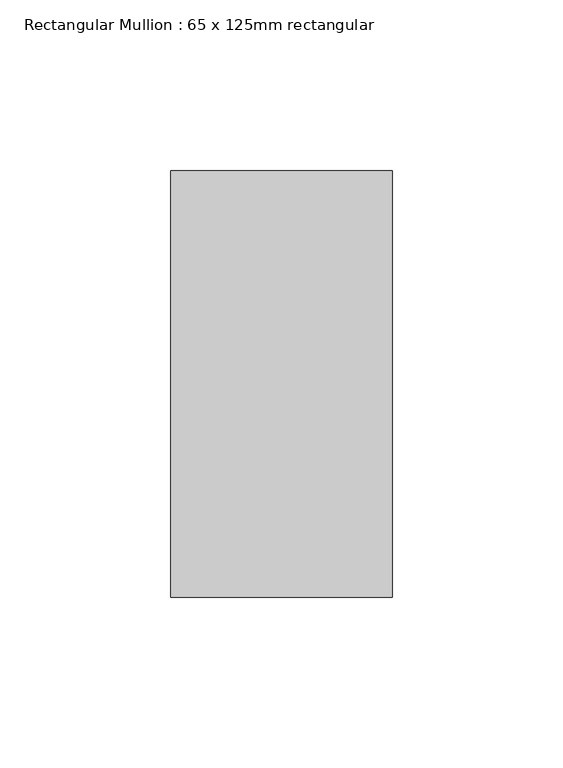
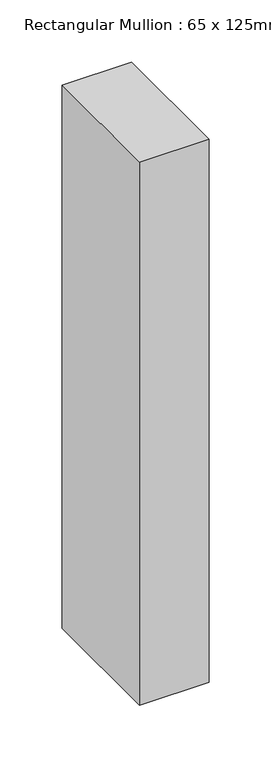
"""IFC4 building model written with IfcOpenShell, lengths in millimetres: member geometry, Rectangular Mullion : 65 x 125mm rectangular."""

from ifc_helpers import new_model, si_unit, frame, origin, place, context, project, spatial, polyline, outline, extrude, source, transform, mapped, element, save


def rectangular_mullion_65_x_125mm_rectangular_3c6cccc9(model_context):
    return source(origin(), model_context, "Body", "SweptSolid", [
        extrude(outline(polyline([(0.0, 62.5), (0.0, -62.5), (-65.0, -62.5), (-65.0, 62.5), (0.0, 62.5)])), frame((0.0, 0.0, -535.0), z_axis=(0.0, 0.0, 1.0), x_axis=(1.0, 0.0, 0.0)), (0.0, 0.0, 1.0), 535.0),
    ])


if __name__ == "__main__":
    model = new_model("IFC4")
    model_context = context("Model", 3, world=origin())
    ifc_project = project(units=[si_unit("LENGTHUNIT", "METRE", prefix="MILLI")], contexts=[model_context])
    site = spatial("IfcSite", under=ifc_project)
    building = spatial("IfcBuilding", under=site)
    placement = place(None, origin())
    rectangular_mullion_65_x_125mm_rectangular_shape = rectangular_mullion_65_x_125mm_rectangular_3c6cccc9(model_context)
    element("IfcMember", 1, ObjectType="Rectangular Mullion : 65 x 125mm rectangular", at=placement, inside=building, context=model_context, shape_type="MappedRepresentation", body=[
        mapped(rectangular_mullion_65_x_125mm_rectangular_shape, transform((0.0, 0.0, 0.0), x_axis=(1.0, 0.0, 0.0), y_axis=(0.0, 1.0, 0.0), z_axis=(0.0, 0.0, 1.0))),
    ])
    save(model, "model.ifc")

# Revit data of these elements
# Type "Rectangular Mullion : 65 x 125mm rectangular"
#   built-in parameter 1007304 = 0.410105 (stored number, unit not read)
#   built-in parameter 1007301 = 0.106627 (stored number, unit not read)
#   built-in parameter 1007300 = 0.106627 (stored number, unit not read)
# Element 1 (IfcMember, "Rectangular Mullion : 65 x 125mm rectangular")
#   Materials on its faces: "Aluminum"
# Materials
#   "Aluminum": class "Metal", colour RGB 244 245 246, transparency 0, Description = "Aluminum 6061", Cost = 0
